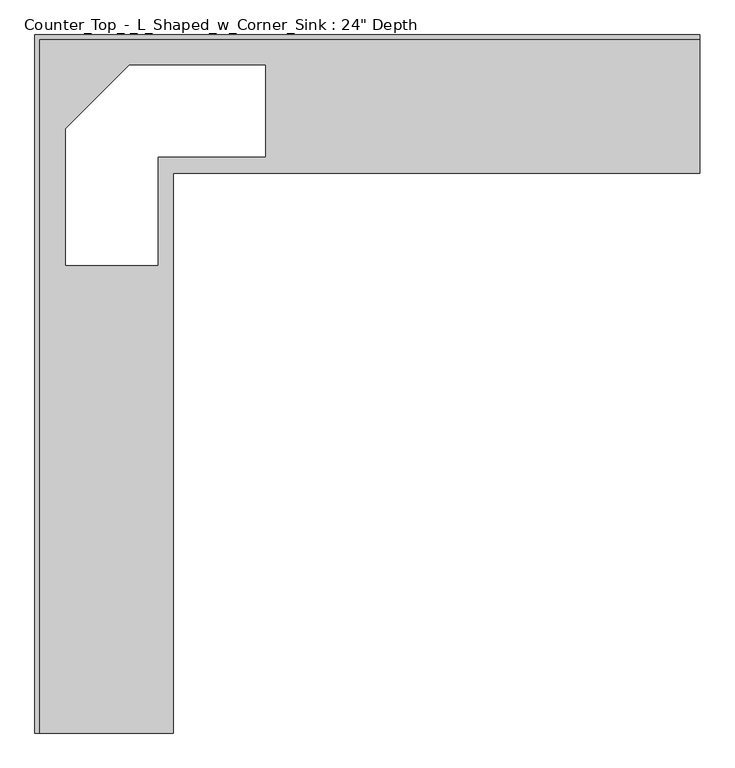
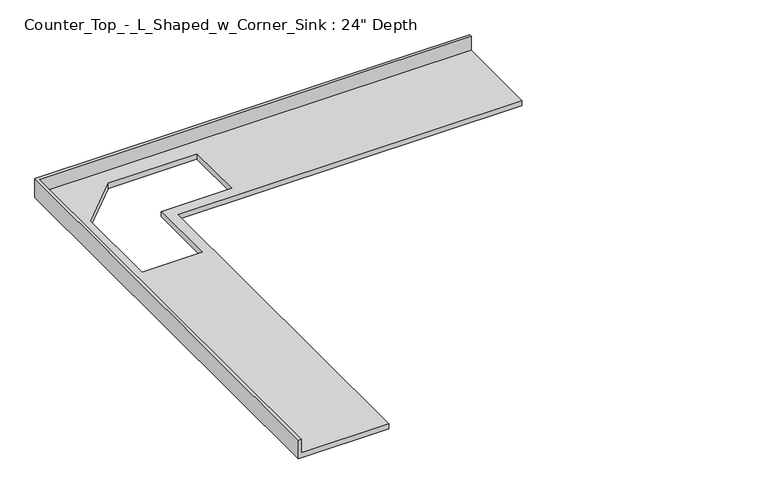
"""IFC4 building model written with IfcOpenShell, lengths in millimetres: furniture geometry."""

from ifc_helpers import new_model, si_unit, origin, place, context, project, spatial, faceted_brep, source, transform, mapped, element, save


def furniture_c73e3426(model_context):
    return source(origin(), model_context, "Body", "Brep", [
        faceted_brep([(-565.4622951, -3200.4, 914.4), (-565.4622951, -635.0, 914.4), (1847.5377049, -635.0, 914.4), (1847.5377049, -19.05, 914.4), (-1181.4122951, -19.05, 914.4), (-1181.4122951, -3200.4, 914.4), (-144.3575457, -559.2047494, 914.4), (-638.3042178, -559.2047494, 914.4), (-638.3042178, -1056.1047494, 914.4), (-1059.0042178, -1056.1047494, 914.4), (-1059.0042178, -430.2384199, 914.4), (-767.2705473, -138.5047494, 914.4), (-144.3575457, -138.5047494, 914.4), (1847.5377049, 0.0, 876.3), (1847.5377049, -635.0, 876.3), (-565.4622951, -635.0, 876.3), (-565.4622951, -3200.4, 876.3), (-1200.4622951, -3200.4, 876.3), (-1200.4622951, 0.0, 876.3), (-144.3575457, -559.2047494, 876.3), (-144.3575457, -138.5047494, 876.3), (-767.2705473, -138.5047494, 876.3), (-1059.0042178, -430.2384199, 876.3), (-1059.0042178, -1056.1047494, 876.3), (-638.3042178, -1056.1047494, 876.3), (-638.3042178, -559.2047494, 876.3), (-1200.4622951, 0.0, 1016.0), (1847.5377049, 0.0, 1016.0), (-1200.4622951, -3200.4, 1016.0), (-1181.4122951, -3200.4, 1016.0), (1847.5377049, -19.05, 1016.0), (-1181.4122951, -19.05, 1016.0)], [[[0, 1, 2, 3, 4, 5], [6, 7, 8, 9, 10, 11, 12]], [[13, 14, 15, 16, 17, 18], [19, 20, 21, 22, 23, 24, 25]], [[13, 18, 26, 27]], [[18, 17, 28, 26]], [[28, 17, 16, 0, 5, 29]], [[1, 0, 16, 15]], [[2, 1, 15, 14]], [[14, 13, 27, 30, 3, 2]], [[7, 6, 19, 25]], [[8, 7, 25, 24]], [[9, 8, 24, 23]], [[10, 9, 23, 22]], [[11, 10, 22, 21]], [[12, 11, 21, 20]], [[6, 12, 20, 19]], [[26, 28, 29, 31, 30, 27]], [[3, 30, 31, 4]], [[31, 29, 5, 4]]]),
    ])


if __name__ == "__main__":
    model = new_model("IFC4")
    model_context = context("Model", 3, world=origin())
    ifc_project = project(units=[si_unit("LENGTHUNIT", "METRE", prefix="MILLI")], contexts=[model_context])
    site = spatial("IfcSite", under=ifc_project)
    building = spatial("IfcBuilding", under=site)
    placement = place(None, origin())
    furniture_shape = furniture_c73e3426(model_context)
    element("IfcFurniture", 1, ObjectType="Counter_Top_-_L_Shaped_w_Corner_Sink : 24\" Depth", at=placement, inside=building, context=model_context, shape_type="MappedRepresentation", body=[
        mapped(furniture_shape, transform((0.0, 0.0, 0.0), x_axis=(1.0, 0.0, 0.0), y_axis=(0.0, 1.0, 0.0), z_axis=(0.0, 0.0, 1.0))),
    ])
    save(model, "model.ifc")

# Revit data of these elements
# Type "Counter_Top_-_L_Shaped_w_Corner_Sink : 24\" Depth"
#   Assembly Code = "C1030400"
#   Sink Opening [instance default] = 1' - 4.56299"
#   Sink Offset (Front) [instance default] = 0' - 2.98406"
#   Counter Thickness = 0' - 1 1/2"
#   Depth = 2' - 1"
#   Height = 3' - 0"
#   Length - Leg 1 [instance default] = 8' - 0"
#   Length - Leg 2 [instance default] = 6' - 0"
#   Counter Top Material = none
#   Default Elevation = 0
# Element 1 (IfcFurniture, "Counter_Top_-_L_Shaped_w_Corner_Sink : 24\" Depth")
#   Length - Leg 1 = 10' - 0"
#   Length - Leg 2 = 10' - 6"
#   Materials on its faces: "Counter Top"
# Materials
#   "Counter Top": colour RGB 226 177 128, transparency 0
